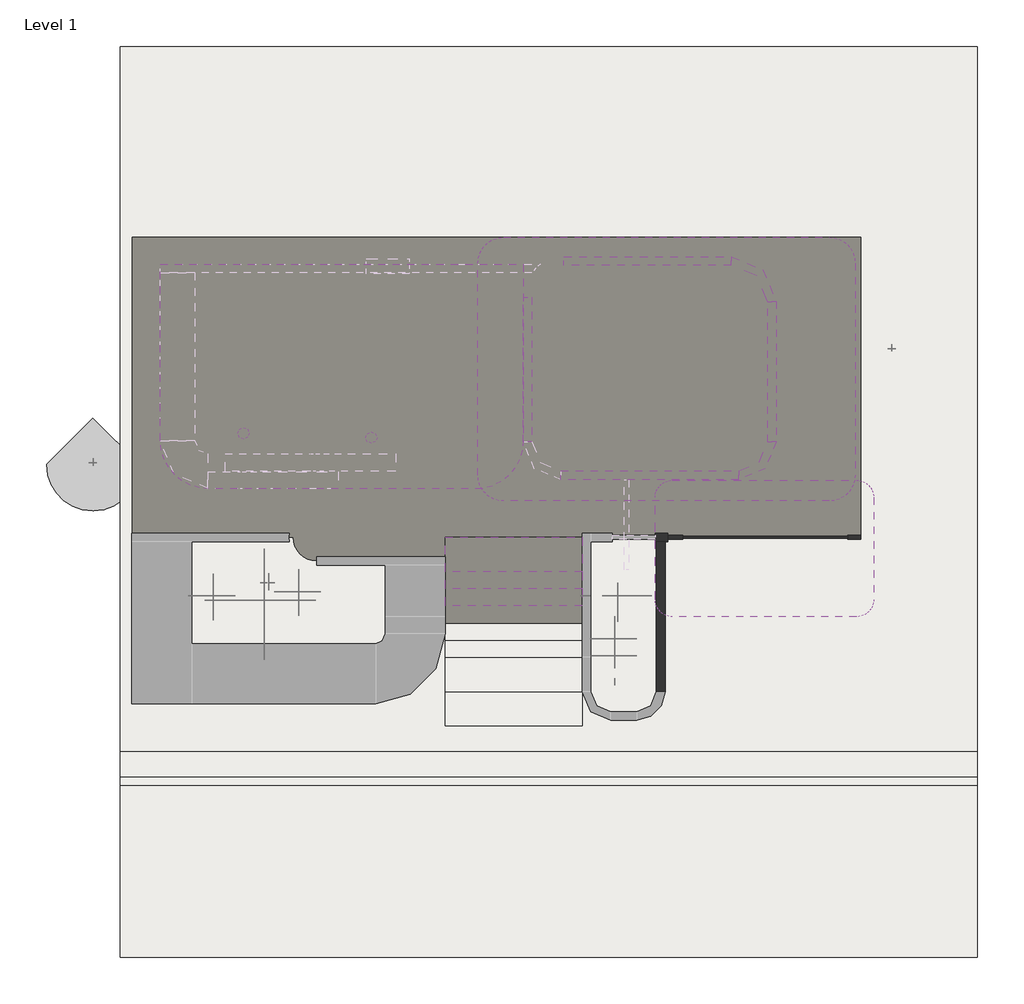
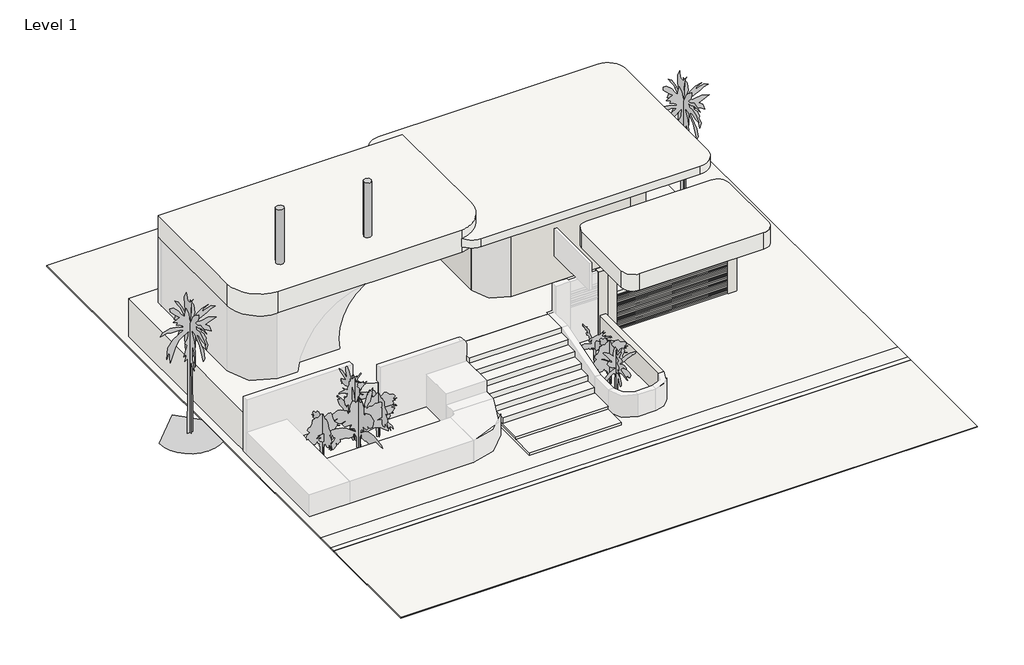
# One storey, part 2 of 2: 16 slabs, 12 walls, 9 geographic elements, 2 columns.
"""IFC4 building model written with IfcOpenShell, lengths in millimetres."""

from ifc_helpers import new_model, si_unit, point, frame, frame_2d, origin, origin_with_axes, place, context, project, spatial, polyline, circle_curve, trimmed, segment, composite_curve, outline, extrude, faceted_brep, transform, mapped, element, save
from components import column_386bdc77, rpc_tree_tropical_d7a905c7, rpc_tree_tropical_australian_tree_furn_6_77f1a640, rpc_tree_tropical_cuban_royal_palm_25_6f0ceb55, rpc_tree_tropical_golden_malay_palm_10_a310d7cf, rpc_tree_tropical_hurricane_palm_12_75f24be5, rpc_tree_tropical_japanese_fiber_banana_8_fc2fb2a9

model = new_model("IFC4")

# Units and contexts
model_context = context("Model", 3, world=origin())
ifc_project = project(units=[si_unit("LENGTHUNIT", "METRE", prefix="MILLI")], contexts=[model_context])

# Site, building, storey
site = spatial("IfcSite", under=ifc_project)
building = spatial("IfcBuilding", under=site)
storey = spatial("IfcBuildingStorey", under=building, Name="Level 1", Elevation=0.0)

# Columns
placement = place(None, origin())
column_shape = column_386bdc77(model_context)
element("IfcColumn", 1, ObjectType="Round Column.0001 : 06\" Diameter", at=placement, inside=storey, context=model_context, shape_type="MappedRepresentation", body=[
    mapped(column_shape, transform((-16218.3035766, 4084.0629979, 0.0), x_axis=(1.0, 0.0, 0.0), y_axis=(0.0, 1.0, 0.0), z_axis=(0.0, 0.0, 1.0))),
])
element("IfcColumn", 2, ObjectType="Round Column.0001 : 06\" Diameter", at=placement, inside=storey, context=model_context, shape_type="MappedRepresentation", body=[
    mapped(column_shape, transform((-11671.7035766, 3931.6629979, 0.0), x_axis=(1.0, 0.0, 0.0), y_axis=(0.0, 1.0, 0.0), z_axis=(0.0, 0.0, 1.0))),
])

# Geographic elements
rpc_tree_tropical_shape = rpc_tree_tropical_d7a905c7(model_context)
element("IfcGeographicElement", 3, ObjectType="RPC Tree - Tropical", at=placement, inside=storey, context=model_context, shape_type="MappedRepresentation", body=[
    mapped(rpc_tree_tropical_shape, transform((-15227.7035766, 3063.3953368, 0.0), x_axis=(1.0, 0.0, 0.0), y_axis=(0.0, 1.0, 0.0), z_axis=(0.0, 0.0, 1.0))),
])
element("IfcGeographicElement", 4, ObjectType="RPC Tree - Tropical", at=placement, inside=storey, context=model_context, shape_type="MappedRepresentation", body=[
    mapped(rpc_tree_tropical_shape, transform((-12179.7035766, 3215.7953368, 0.0), x_axis=(1.0, 0.0, 0.0), y_axis=(0.0, 1.0, 0.0), z_axis=(0.0, 0.0, 1.0))),
])
element("IfcGeographicElement", 5, ObjectType="RPC Tree - Tropical", at=placement, inside=storey, context=model_context, shape_type="MappedRepresentation", body=[
    mapped(rpc_tree_tropical_shape, transform((-936.864807, 1539.3953368, 0.0), x_axis=(1.0, 0.0, 0.0), y_axis=(0.0, 1.0, 0.0), z_axis=(0.0, 0.0, 1.0))),
])
rpc_tree_tropical_australian_tree_furn_6_shape = rpc_tree_tropical_australian_tree_furn_6_77f1a640(model_context)
element("IfcGeographicElement", 6, ObjectType="RPC Tree - Tropical : Australian Tree Furn - 6'", at=placement, inside=storey, context=model_context, shape_type="MappedRepresentation", body=[
    mapped(rpc_tree_tropical_australian_tree_furn_6_shape, transform((-828.8944013, 3063.3953368, 0.0), x_axis=(1.0, 0.0, 0.0), y_axis=(0.0, 1.0, 0.0), z_axis=(0.0, 0.0, 1.0))),
])
rpc_tree_tropical_cuban_royal_palm_25_shape = rpc_tree_tropical_cuban_royal_palm_25_6f0ceb55(model_context)
element("IfcGeographicElement", 7, ObjectType="RPC Tree - Tropical : Cuban Royal Palm - 25'", at=placement, inside=storey, context=model_context, shape_type="MappedRepresentation", body=[
    mapped(rpc_tree_tropical_cuban_royal_palm_25_shape, transform((-19494.9035766, 7787.7953368, 0.0), x_axis=(1.0, 0.0, 0.0), y_axis=(0.0, 1.0, 0.0), z_axis=(0.0, 0.0, 1.0))),
])
element("IfcGeographicElement", 8, ObjectType="RPC Tree - Tropical : Cuban Royal Palm - 25'", at=placement, inside=storey, context=model_context, shape_type="MappedRepresentation", body=[
    mapped(rpc_tree_tropical_cuban_royal_palm_25_shape, transform((8914.5561229, 11850.2999244, 0.0), x_axis=(1.0, 0.0, 0.0), y_axis=(0.0, 1.0, 0.0), z_axis=(0.0, 0.0, 1.0))),
])
rpc_tree_tropical_golden_malay_palm_10_shape = rpc_tree_tropical_golden_malay_palm_10_a310d7cf(model_context)
element("IfcGeographicElement", 9, ObjectType="RPC Tree - Tropical : Golden Malay Palm - 10'", at=placement, inside=storey, context=model_context, shape_type="MappedRepresentation", body=[
    mapped(rpc_tree_tropical_golden_malay_palm_10_shape, transform((-13398.9035766, 2910.9953368, 0.0), x_axis=(1.0, 0.0, 0.0), y_axis=(0.0, 1.0, 0.0), z_axis=(0.0, 0.0, 1.0))),
])
rpc_tree_tropical_hurricane_palm_12_shape = rpc_tree_tropical_hurricane_palm_12_75f24be5(model_context)
element("IfcGeographicElement", 10, ObjectType="RPC Tree - Tropical : Hurricane Palm - 12'", at=placement, inside=storey, context=model_context, shape_type="MappedRepresentation", body=[
    mapped(rpc_tree_tropical_hurricane_palm_12_shape, transform((-13246.5035766, 3520.5953368, 0.0), x_axis=(1.0, 0.0, 0.0), y_axis=(0.0, 1.0, 0.0), z_axis=(0.0, 0.0, 1.0))),
])
rpc_tree_tropical_japanese_fiber_banana_8_shape = rpc_tree_tropical_japanese_fiber_banana_8_fc2fb2a9(model_context)
element("IfcGeographicElement", 11, ObjectType="RPC Tree - Tropical : Japanese Fiber Banana - 8'", at=placement, inside=storey, context=model_context, shape_type="MappedRepresentation", body=[
    mapped(rpc_tree_tropical_japanese_fiber_banana_8_shape, transform((-936.864807, 929.7953368, 0.0), x_axis=(1.0, 0.0, 0.0), y_axis=(0.0, 1.0, 0.0), z_axis=(0.0, 0.0, 1.0))),
])

# Slabs
element("IfcSlab", 12, ObjectType="Generic - 1.5'", at=placement, inside=storey, context=model_context, shape_type="SweptSolid", body=[
    extrude(outline(composite_curve([segment(trimmed(circle_curve(frame_2d((6692.4964234, 14898.2999244)), 914.4), [point((6692.4964234, 15812.6999244))], [point((7606.8964234, 14898.2999244))], False, "CARTESIAN"), True, "CONTINUOUS"), segment(polyline([(7606.8964234, 14898.2999244), (7606.8964234, 7349.8857607)]), True, "CONTINUOUS"), segment(trimmed(circle_curve(frame_2d((6692.4964234, 7349.8857607)), 914.4), [point((7606.8964234, 7349.8857607))], [point((6692.4964234, 6435.4857607))], False, "CARTESIAN"), True, "CONTINUOUS"), segment(polyline([(6692.4964234, 6435.4857607), (-4890.8055301, 6435.4857607)]), True, "CONTINUOUS"), segment(trimmed(circle_curve(frame_2d((-4890.8055301, 7349.8857607)), 914.4), [point((-4890.8055301, 6435.4857607))], [point((-5805.2055301, 7349.8857607))], False, "CARTESIAN"), True, "CONTINUOUS"), segment(polyline([(-5805.2055301, 7349.8857607), (-5805.2055301, 14898.2999244)]), True, "CONTINUOUS"), segment(trimmed(circle_curve(frame_2d((-4890.8055301, 14898.2999244)), 914.4), [point((-5805.2055301, 14898.2999244))], [point((-4890.8055301, 15812.6999244))], False, "CARTESIAN"), True, "CONTINUOUS"), segment(polyline([(-4890.8055301, 15812.6999244), (6692.4964234, 15812.6999244)]), True, "CONTINUOUS")], self_intersect=False)), frame((0.0, 0.0, 6096.0), z_axis=(0.0, 0.0, 1.0), x_axis=(1.0, 0.0, 0.0)), (0.0, 0.0, 1.0), 457.2),
])
element("IfcSlab", 13, ObjectType="Generic - 12\"", at=placement, inside=storey, context=model_context, shape_type="SweptSolid", body=[
    extrude(outline(polyline([(-2097.7074836, 5144.6999244), (-2097.7074836, 877.4999244), (-6974.5074836, 877.4999244), (-6974.5074836, 5144.6999244), (-2097.7074836, 5144.6999244)])), frame((0.0, 0.0, 304.8), z_axis=(0.0, 0.0, 1.0), x_axis=(1.0, 0.0, 0.0)), (0.0, 0.0, 1.0), 304.8),
])
element("IfcSlab", 14, ObjectType="Generic - 12\"", at=placement, inside=storey, context=model_context, shape_type="SweptSolid", body=[
    extrude(outline(polyline([(-2097.7074836, 5144.6999244), (-2097.7074836, 1487.0999244), (-6974.5074836, 1487.0999244), (-6974.5074836, 5144.6999244), (-2097.7074836, 5144.6999244)])), frame((0.0, 0.0, 609.6), z_axis=(0.0, 0.0, 1.0), x_axis=(1.0, 0.0, 0.0)), (0.0, 0.0, 1.0), 304.8),
])
element("IfcSlab", 15, ObjectType="Generic - 12\"", at=placement, inside=storey, context=model_context, shape_type="SweptSolid", body=[
    extrude(outline(polyline([(-2097.7074836, 5144.6999244), (-2097.7074836, 2096.6999244), (-6974.5074836, 2096.6999244), (-6974.5074836, 5144.6999244), (-2097.7074836, 5144.6999244)])), frame((0.0, 0.0, 914.4), z_axis=(0.0, 0.0, 1.0), x_axis=(1.0, 0.0, 0.0)), (0.0, 0.0, 1.0), 304.8),
])
element("IfcSlab", 16, ObjectType="Generic - 12\"", at=placement, inside=storey, context=model_context, shape_type="SweptSolid", body=[
    extrude(outline(polyline([(-2097.7074836, 5144.6999244), (-2097.7074836, 2706.3092226), (-6974.5074836, 2706.3092226), (-6974.5074836, 5144.6999244), (-2097.7074836, 5144.6999244)])), frame((0.0, 0.0, 1219.2), z_axis=(0.0, 0.0, 1.0), x_axis=(1.0, 0.0, 0.0)), (0.0, 0.0, 1.0), 304.8),
])
element("IfcSlab", 17, ObjectType="Generic - 12\"", at=placement, inside=storey, context=model_context, shape_type="SweptSolid", body=[
    extrude(outline(polyline([(-2097.7074836, 5144.6999244), (-2097.7074836, 3315.8999244), (-6974.5074836, 3315.8999244), (-6974.5074836, 5144.6999244), (-2097.7074836, 5144.6999244)])), frame((0.0, 0.0, 1524.0), z_axis=(0.0, 0.0, 1.0), x_axis=(1.0, 0.0, 0.0)), (0.0, 0.0, 1.0), 304.8),
])
element("IfcSlab", 18, ObjectType="Generic - 12\"", at=placement, inside=storey, context=model_context, shape_type="SweptSolid", body=[
    extrude(outline(polyline([(-2097.7074836, 5144.6999244), (-2097.7074836, 3925.5045735), (-6974.5074836, 3925.5045735), (-6974.5074836, 5144.6999244), (-2097.7074836, 5144.6999244)])), frame((0.0, 0.0, 1828.8), z_axis=(0.0, 0.0, 1.0), x_axis=(1.0, 0.0, 0.0)), (0.0, 0.0, 1.0), 304.8),
])
element("IfcSlab", 19, ObjectType="Generic - 2\"", at=placement, inside=storey, context=model_context, shape_type="SweptSolid", body=[
    extrude(outline(polyline([(11957.1530585, 22597.74911), (11957.1530585, -2475.3000756), (-18522.8469415, -2475.3000756), (-18522.8469415, 22597.74911), (11957.1530585, 22597.74911)])), frame((0.0, 0.0, -50.8), z_axis=(0.0, 0.0, 1.0), x_axis=(1.0, 0.0, 0.0)), (0.0, 0.0, 1.0), 50.8),
])
element("IfcSlab", 20, ObjectType="Generic - 2\" gray", at=placement, inside=storey, context=model_context, shape_type="SweptSolid", body=[
    extrude(outline(polyline([(-18522.8469415, -2475.3000756), (11957.1530585, -2475.3000756), (11957.1530585, -3389.7000756), (-18522.8469415, -3389.7000756), (-18522.8469415, -2475.3000756)])), frame((0.0, 0.0, -50.8), z_axis=(0.0, 0.0, 1.0), x_axis=(1.0, 0.0, 0.0)), (0.0, 0.0, 1.0), 50.8),
])
element("IfcSlab", 21, ObjectType="Generic - 2\" gray", at=placement, inside=storey, context=model_context, shape_type="SweptSolid", body=[
    extrude(outline(polyline([(-18522.8469415, -3694.5000756), (11957.1530585, -3694.5000756), (11957.1530585, -9790.5000756), (-18522.8469415, -9790.5000756), (-18522.8469415, -3694.5000756)])), frame((0.0, 0.0, -50.8), z_axis=(0.0, 0.0, 1.0), x_axis=(1.0, 0.0, 0.0)), (0.0, 0.0, 1.0), 50.8),
])
element("IfcSlab", 22, ObjectType="Generic - 2\" white", at=placement, inside=storey, context=model_context, shape_type="SweptSolid", body=[
    extrude(outline(polyline([(-18522.8469415, -3389.7000756), (11957.1530585, -3389.7000756), (11957.1530585, -3694.5000756), (-18522.8469415, -3694.5000756), (-18522.8469415, -3389.7000756)])), frame((0.0, 0.0, -50.8), z_axis=(0.0, 0.0, 1.0), x_axis=(1.0, 0.0, 0.0)), (0.0, 0.0, 1.0), 50.8),
])
element("IfcSlab", 23, ObjectType="Generic - 3'", at=placement, inside=storey, context=model_context, shape_type="SweptSolid", body=[
    extrude(outline(composite_curve([segment(trimmed(circle_curve(frame_2d((7657.6964234, 6562.4857607)), 609.6), [point((7657.6964234, 7172.0857607))], [point((8267.2964234, 6562.4857607))], False, "CARTESIAN"), True, "CONTINUOUS"), segment(polyline([(8267.2964234, 6562.4857607), (8267.2964234, 2927.6793884)]), True, "CONTINUOUS"), segment(trimmed(circle_curve(frame_2d((7657.6964234, 2927.6793884)), 609.6), [point((8267.2964234, 2927.6793884))], [point((7657.6964234, 2318.0793884))], False, "CARTESIAN"), True, "CONTINUOUS"), segment(polyline([(7657.6964234, 2318.0793884), (1104.4964234, 2318.0793884)]), True, "CONTINUOUS"), segment(trimmed(circle_curve(frame_2d((1104.4964234, 2927.6793884)), 609.6), [point((1104.4964234, 2318.0793884))], [point((494.8964234, 2927.6793884))], False, "CARTESIAN"), True, "CONTINUOUS"), segment(polyline([(494.8964234, 2927.6793884), (494.8964234, 6562.4857607)]), True, "CONTINUOUS"), segment(trimmed(circle_curve(frame_2d((1104.4964234, 6562.4857607)), 609.6), [point((494.8964234, 6562.4857607))], [point((1104.4964234, 7172.0857607))], False, "CARTESIAN"), True, "CONTINUOUS"), segment(polyline([(1104.4964234, 7172.0857607), (7657.6964234, 7172.0857607)]), True, "CONTINUOUS")], self_intersect=False)), frame((0.0, 0.0, 4064.0), z_axis=(0.0, 0.0, 1.0), x_axis=(1.0, 0.0, 0.0)), (0.0, 0.0, 1.0), 914.4),
])
element("IfcSlab", 24, ObjectType="Generic - 3.5'", at=placement, inside=storey, context=model_context, shape_type="SweptSolid", body=[
    extrude(outline(composite_curve([segment(polyline([(-18097.9035766, 15812.6999244), (7808.2925164, 15812.6999244), (7808.2925164, 5144.6999244), (-6974.5074836, 5144.6999244), (-6974.5074836, 4309.74911), (-11546.5074836, 4309.74911)]), True, "CONTINUOUS"), segment(trimmed(circle_curve(frame_2d((-11546.5074836, 5144.6999244)), 834.9508144), [point((-11546.5074836, 4309.74911))], [point((-12381.458298, 5144.6999244))], False, "CARTESIAN"), True, "CONTINUOUS"), segment(polyline([(-12381.458298, 5144.6999244), (-18097.9035766, 5144.6999244), (-18097.9035766, 15812.6999244)]), True, "CONTINUOUS")], self_intersect=False)), origin_with_axes(), (0.0, 0.0, 1.0), 2133.6),
])
element("IfcSlab", 25, ObjectType="Generic - 5'", at=placement, inside=storey, context=model_context, shape_type="SweptSolid", body=[
    extrude(outline(composite_curve([segment(polyline([(-17097.1000691, 8579.8629979), (-17097.1000691, 14853.6629979), (-4191.8438771, 14853.6629979), (-4191.8438771, 8579.8629979)]), True, "CONTINUOUS"), segment(trimmed(circle_curve(frame_2d((-5921.3536308, 8579.8629979)), 1729.5097537), [point((-4191.8438771, 8579.8629979))], [point((-5637.4510356, 6873.8139644))], False, "CARTESIAN"), True, "CONTINUOUS"), segment(polyline([(-5637.4510356, 6873.8139644), (-15391.0510356, 6873.8139644)]), True, "CONTINUOUS"), segment(trimmed(circle_curve(frame_2d((-15391.0510356, 8579.8629979)), 1706.0490335), [point((-15391.0510356, 6873.8139644))], [point((-17097.1000691, 8579.8629979))], False, "CARTESIAN"), True, "CONTINUOUS")], self_intersect=False)), frame((0.0, 0.0, 5791.2), z_axis=(0.0, 0.0, 1.0), x_axis=(1.0, 0.0, 0.0)), (0.0, 0.0, 1.0), 1219.2),
])
element("IfcSlab", 26, ObjectType="Generic - 6\"", at=placement, inside=storey, context=model_context, shape_type="SweptSolid", body=[
    extrude(outline(polyline([(-2097.7074836, 5144.6999244), (-2097.7074836, -1560.9000756), (-6974.5074836, -1560.9000756), (-6974.5074836, 5144.6999244), (-2097.7074836, 5144.6999244)])), origin_with_axes(), (0.0, 0.0, 1.0), 152.4),
])
element("IfcSlab", 27, ObjectType="Generic - 6\"", at=placement, inside=storey, context=model_context, shape_type="SweptSolid", body=[
    extrude(outline(polyline([(-2097.7074836, 5144.6999244), (-2097.7074836, -341.7000756), (-6974.5074836, -341.7000756), (-6974.5074836, 5144.6999244), (-2097.7074836, 5144.6999244)])), frame((0.0, 0.0, 152.4), z_axis=(0.0, 0.0, 1.0), x_axis=(1.0, 0.0, 0.0)), (0.0, 0.0, 1.0), 152.4),
])

# Walls
element("IfcWall", 28, ObjectType="Generic - 12\" white", at=placement, inside=storey, context=model_context, shape_type="SweptSolid", body=[
    extrude(outline(polyline([(847.5055987, 4992.2999244), (847.5055987, -341.7000756), (542.7055987, -341.7000756), (542.7055987, 4992.2999244), (847.5055987, 4992.2999244)])), origin_with_axes(), (0.0, 0.0, 1.0), 1219.2),
])
element("IfcWall", 29, ObjectType="Generic - 12\" white", at=placement, inside=storey, context=model_context, shape_type="Brep", body=[
    faceted_brep([(494.8964234, 4992.2999244, 3657.6), (494.8964234, 4992.2999244, 0.0), (542.7055987, 4992.2999244, 0.0), (847.5055987, 4992.2999244, 0.0), (952.0964234, 4992.2999244, 0.0), (952.0964234, 4992.2999244, 3657.6), (494.8964234, 5297.0999244, 0.0), (494.8964234, 5297.0999244, 3657.6), (952.0964234, 5297.0999244, 3657.6), (952.0964234, 5297.0999244, 0.0), (494.8964234, 5068.4999244, 0.0), (494.8964234, 5220.8999244, 0.0), (952.0964234, 5220.8999244, 0.0), (952.0964234, 5068.4999244, 0.0)], [[[0, 1, 2, 3, 4, 5]], [[6, 7, 8, 9]], [[4, 3, 2, 1, 10, 11, 6, 9, 12, 13]], [[5, 4, 13, 12, 9, 8]], [[0, 5, 8, 7]], [[0, 7, 6, 11, 10, 1]]]),
])
element("IfcWall", 30, ObjectType="Generic - 12\" white", at=placement, inside=storey, context=model_context, shape_type="SweptSolid", body=[
    extrude(outline(polyline([(-3887.0438771, 13679.0999244), (-3887.0438771, 8537.6506138), (-4191.8438771, 8537.6506138), (-4191.8438771, 13679.0999244), (-3887.0438771, 13679.0999244)])), frame((0.0, 0.0, 2133.6), z_axis=(0.0, 0.0, 1.0), x_axis=(1.0, 0.0, 0.0)), (0.0, 0.0, 1.0), 3657.6),
])
element("IfcWall", 31, ObjectType="Generic - 12\" white", at=placement, inside=storey, context=model_context, shape_type="SweptSolid", body=[
    extrude(outline(polyline([(4494.9561229, 8537.6506138), (4494.9561229, 13522.2136873), (4799.7561229, 13522.2136873), (4799.7561229, 8537.6506138), (4494.9561229, 8537.6506138)])), frame((0.0, 0.0, 2133.6), z_axis=(0.0, 0.0, 1.0), x_axis=(1.0, 0.0, 0.0)), (0.0, 0.0, 1.0), 3962.4),
])
element("IfcWall", 32, ObjectType="Generic - 12\" white", at=placement, inside=storey, context=model_context, shape_type="SweptSolid", body=[
    extrude(outline(polyline([(-2746.2869957, 15124.6568058), (3197.3130043, 15124.6568058), (3197.3130043, 14819.8568058), (-2746.2869957, 14819.8568058), (-2746.2869957, 15124.6568058)])), frame((0.0, 0.0, 2133.6), z_axis=(0.0, 0.0, 1.0), x_axis=(1.0, 0.0, 0.0)), (0.0, 0.0, 1.0), 3962.4),
])
element("IfcWall", 33, ObjectType="Generic - 12\" white", at=placement, inside=storey, context=model_context, shape_type="SweptSolid", body=[
    extrude(outline(composite_curve([segment(polyline([(3461.9623149, 7199.8568058), (3461.9623149, 7504.6568058)]), True, "CONTINUOUS"), segment(trimmed(circle_curve(frame_2d((3461.9623149, 8537.6506138)), 1032.993808), [point((3461.9623149, 7504.6568058))], [point((4494.9561229, 8537.6506138))], True, "CARTESIAN"), True, "CONTINUOUS"), segment(polyline([(4494.9561229, 8537.6506138), (4799.7561229, 8537.6506138)]), True, "CONTINUOUS"), segment(trimmed(circle_curve(frame_2d((3461.9623149, 8537.6506138)), 1337.793808), [point((4799.7561229, 8537.6506138))], [point((3461.9623149, 7199.8568058))], False, "CARTESIAN"), True, "CONTINUOUS")], self_intersect=False)), frame((0.0, 0.0, 2133.6), z_axis=(0.0, 0.0, 1.0), x_axis=(1.0, 0.0, 0.0)), (0.0, 0.0, 1.0), 3962.4),
])
element("IfcWall", 34, ObjectType="Generic - 12\" white", at=placement, inside=storey, context=model_context, shape_type="SweptSolid", body=[
    extrude(outline(polyline([(-2854.0500691, 7504.6568058), (3461.9623149, 7504.6568058), (3461.9623149, 7199.8568058), (-2854.0500691, 7199.8568058), (-2854.0500691, 7504.6568058)])), frame((0.0, 0.0, 2133.6), z_axis=(0.0, 0.0, 1.0), x_axis=(1.0, 0.0, 0.0)), (0.0, 0.0, 1.0), 3962.4),
])
element("IfcWall", 35, ObjectType="Generic - 12\" white", at=placement, inside=storey, context=model_context, shape_type="SweptSolid", body=[
    extrude(outline(composite_curve([segment(polyline([(4799.7561229, 13522.2136873), (4494.9561229, 13522.2136873)]), True, "CONTINUOUS"), segment(trimmed(circle_curve(frame_2d((3197.3130043, 13522.2136873)), 1297.6431186), [point((4494.9561229, 13522.2136873))], [point((3197.3130043, 14819.8568058))], True, "CARTESIAN"), True, "CONTINUOUS"), segment(polyline([(3197.3130043, 14819.8568058), (3197.3130043, 15124.6568058)]), True, "CONTINUOUS"), segment(trimmed(circle_curve(frame_2d((3197.3130043, 13522.2136873)), 1602.4431186), [point((3197.3130043, 15124.6568058))], [point((4799.7561229, 13522.2136873))], False, "CARTESIAN"), True, "CONTINUOUS")], self_intersect=False)), frame((0.0, 0.0, 2133.6), z_axis=(0.0, 0.0, 1.0), x_axis=(1.0, 0.0, 0.0)), (0.0, 0.0, 1.0), 3962.4),
])
element("IfcWall", 36, ObjectType="Generic - 3\" white 2", at=placement, inside=storey, context=model_context, shape_type="SweptSolid", body=[
    extrude(outline(polyline([(7352.8964234, 5106.5999244), (1468.8829427, 5106.5999244), (1468.8829427, 5182.7999244), (7352.8964234, 5182.7999244), (7352.8964234, 5106.5999244)])), origin_with_axes(), (0.0, 0.0, 1.0), 76.2),
    extrude(outline(polyline([(7352.8964234, 5106.5999244), (1468.8829427, 5106.5999244), (1468.8829427, 5182.7999244), (7352.8964234, 5182.7999244), (7352.8964234, 5106.5999244)])), frame((0.0, 0.0, 88.9), z_axis=(0.0, 0.0, 1.0), x_axis=(1.0, 0.0, 0.0)), (0.0, 0.0, 1.0), 76.2),
    extrude(outline(polyline([(7352.8964234, 5106.5999244), (1468.8829427, 5106.5999244), (1468.8829427, 5182.7999244), (7352.8964234, 5182.7999244), (7352.8964234, 5106.5999244)])), frame((0.0, 0.0, 177.8), z_axis=(0.0, 0.0, 1.0), x_axis=(1.0, 0.0, 0.0)), (0.0, 0.0, 1.0), 76.2),
    extrude(outline(polyline([(7352.8964234, 5106.5999244), (1468.8829427, 5106.5999244), (1468.8829427, 5182.7999244), (7352.8964234, 5182.7999244), (7352.8964234, 5106.5999244)])), frame((0.0, 0.0, 266.7), z_axis=(0.0, 0.0, 1.0), x_axis=(1.0, 0.0, 0.0)), (0.0, 0.0, 1.0), 76.2),
    extrude(outline(polyline([(7352.8964234, 5106.5999244), (1468.8829427, 5106.5999244), (1468.8829427, 5182.7999244), (7352.8964234, 5182.7999244), (7352.8964234, 5106.5999244)])), frame((0.0, 0.0, 355.6), z_axis=(0.0, 0.0, 1.0), x_axis=(1.0, 0.0, 0.0)), (0.0, 0.0, 1.0), 76.2),
    extrude(outline(polyline([(7352.8964234, 5106.5999244), (1468.8829427, 5106.5999244), (1468.8829427, 5182.7999244), (7352.8964234, 5182.7999244), (7352.8964234, 5106.5999244)])), frame((0.0, 0.0, 444.5), z_axis=(0.0, 0.0, 1.0), x_axis=(1.0, 0.0, 0.0)), (0.0, 0.0, 1.0), 76.2),
    extrude(outline(polyline([(7352.8964234, 5106.5999244), (1468.8829427, 5106.5999244), (1468.8829427, 5182.7999244), (7352.8964234, 5182.7999244), (7352.8964234, 5106.5999244)])), frame((0.0, 0.0, 533.4), z_axis=(0.0, 0.0, 1.0), x_axis=(1.0, 0.0, 0.0)), (0.0, 0.0, 1.0), 76.2),
    extrude(outline(polyline([(7352.8964234, 5106.5999244), (1468.8829427, 5106.5999244), (1468.8829427, 5182.7999244), (7352.8964234, 5182.7999244), (7352.8964234, 5106.5999244)])), frame((0.0, 0.0, 622.3), z_axis=(0.0, 0.0, 1.0), x_axis=(1.0, 0.0, 0.0)), (0.0, 0.0, 1.0), 76.2),
    extrude(outline(polyline([(7352.8964234, 5106.5999244), (1468.8829427, 5106.5999244), (1468.8829427, 5182.7999244), (7352.8964234, 5182.7999244), (7352.8964234, 5106.5999244)])), frame((0.0, 0.0, 711.2), z_axis=(0.0, 0.0, 1.0), x_axis=(1.0, 0.0, 0.0)), (0.0, 0.0, 1.0), 76.2),
    extrude(outline(polyline([(7352.8964234, 5106.5999244), (1468.8829427, 5106.5999244), (1468.8829427, 5182.7999244), (7352.8964234, 5182.7999244), (7352.8964234, 5106.5999244)])), frame((0.0, 0.0, 800.1), z_axis=(0.0, 0.0, 1.0), x_axis=(1.0, 0.0, 0.0)), (0.0, 0.0, 1.0), 76.2),
    extrude(outline(polyline([(7352.8964234, 5106.5999244), (1468.8829427, 5106.5999244), (1468.8829427, 5182.7999244), (7352.8964234, 5182.7999244), (7352.8964234, 5106.5999244)])), frame((0.0, 0.0, 889.0), z_axis=(0.0, 0.0, 1.0), x_axis=(1.0, 0.0, 0.0)), (0.0, 0.0, 1.0), 76.2),
])
element("IfcWall", 37, ObjectType="Generic - 3\" white 2", at=placement, inside=storey, context=model_context, shape_type="SweptSolid", body=[
    extrude(outline(polyline([(7352.8964234, 5106.5999244), (1468.8829427, 5106.5999244), (1468.8829427, 5182.7999244), (7352.8964234, 5182.7999244), (7352.8964234, 5106.5999244)])), frame((0.0, 0.0, 987.425), z_axis=(0.0, 0.0, 1.0), x_axis=(1.0, 0.0, 0.0)), (0.0, 0.0, 1.0), 76.2),
    extrude(outline(polyline([(7352.8964234, 5106.5999244), (1468.8829427, 5106.5999244), (1468.8829427, 5182.7999244), (7352.8964234, 5182.7999244), (7352.8964234, 5106.5999244)])), frame((0.0, 0.0, 1076.325), z_axis=(0.0, 0.0, 1.0), x_axis=(1.0, 0.0, 0.0)), (0.0, 0.0, 1.0), 76.2),
    extrude(outline(polyline([(7352.8964234, 5106.5999244), (1468.8829427, 5106.5999244), (1468.8829427, 5182.7999244), (7352.8964234, 5182.7999244), (7352.8964234, 5106.5999244)])), frame((0.0, 0.0, 1165.225), z_axis=(0.0, 0.0, 1.0), x_axis=(1.0, 0.0, 0.0)), (0.0, 0.0, 1.0), 76.2),
    extrude(outline(polyline([(7352.8964234, 5106.5999244), (1468.8829427, 5106.5999244), (1468.8829427, 5182.7999244), (7352.8964234, 5182.7999244), (7352.8964234, 5106.5999244)])), frame((0.0, 0.0, 1254.125), z_axis=(0.0, 0.0, 1.0), x_axis=(1.0, 0.0, 0.0)), (0.0, 0.0, 1.0), 76.2),
    extrude(outline(polyline([(7352.8964234, 5106.5999244), (1468.8829427, 5106.5999244), (1468.8829427, 5182.7999244), (7352.8964234, 5182.7999244), (7352.8964234, 5106.5999244)])), frame((0.0, 0.0, 1343.025), z_axis=(0.0, 0.0, 1.0), x_axis=(1.0, 0.0, 0.0)), (0.0, 0.0, 1.0), 76.2),
    extrude(outline(polyline([(7352.8964234, 5106.5999244), (1468.8829427, 5106.5999244), (1468.8829427, 5182.7999244), (7352.8964234, 5182.7999244), (7352.8964234, 5106.5999244)])), frame((0.0, 0.0, 1431.925), z_axis=(0.0, 0.0, 1.0), x_axis=(1.0, 0.0, 0.0)), (0.0, 0.0, 1.0), 76.2),
    extrude(outline(polyline([(7352.8964234, 5106.5999244), (1468.8829427, 5106.5999244), (1468.8829427, 5182.7999244), (7352.8964234, 5182.7999244), (7352.8964234, 5106.5999244)])), frame((0.0, 0.0, 1520.825), z_axis=(0.0, 0.0, 1.0), x_axis=(1.0, 0.0, 0.0)), (0.0, 0.0, 1.0), 76.2),
    extrude(outline(polyline([(7352.8964234, 5106.5999244), (1468.8829427, 5106.5999244), (1468.8829427, 5182.7999244), (7352.8964234, 5182.7999244), (7352.8964234, 5106.5999244)])), frame((0.0, 0.0, 1609.725), z_axis=(0.0, 0.0, 1.0), x_axis=(1.0, 0.0, 0.0)), (0.0, 0.0, 1.0), 76.2),
    extrude(outline(polyline([(7352.8964234, 5106.5999244), (1468.8829427, 5106.5999244), (1468.8829427, 5182.7999244), (7352.8964234, 5182.7999244), (7352.8964234, 5106.5999244)])), frame((0.0, 0.0, 1698.625), z_axis=(0.0, 0.0, 1.0), x_axis=(1.0, 0.0, 0.0)), (0.0, 0.0, 1.0), 76.2),
    extrude(outline(polyline([(7352.8964234, 5106.5999244), (1468.8829427, 5106.5999244), (1468.8829427, 5182.7999244), (7352.8964234, 5182.7999244), (7352.8964234, 5106.5999244)])), frame((0.0, 0.0, 1787.525), z_axis=(0.0, 0.0, 1.0), x_axis=(1.0, 0.0, 0.0)), (0.0, 0.0, 1.0), 76.2),
    extrude(outline(polyline([(7352.8964234, 5106.5999244), (1468.8829427, 5106.5999244), (1468.8829427, 5182.7999244), (7352.8964234, 5182.7999244), (7352.8964234, 5106.5999244)])), frame((0.0, 0.0, 1876.425), z_axis=(0.0, 0.0, 1.0), x_axis=(1.0, 0.0, 0.0)), (0.0, 0.0, 1.0), 76.2),
])
element("IfcWall", 38, ObjectType="Generic - 6\" white", at=placement, inside=storey, context=model_context, shape_type="Brep", body=[
    faceted_brep([(952.0964234, 5068.4999244, 0.0), (1468.8829427, 5068.4999244, 0.0), (1468.8829427, 5068.4999244, 4876.8), (952.0964234, 5068.4999244, 4876.8), (952.0964234, 5220.8999244, 0.0), (952.0964234, 5220.8999244, 4876.8), (1468.8829427, 5220.8999244, 4876.8), (1468.8829427, 5220.8999244, 0.0), (1468.8829427, 5182.7999244, 0.0), (1468.8829427, 5106.5999244, 0.0)], [[[0, 1, 2, 3]], [[4, 5, 6, 7]], [[1, 0, 4, 7, 8, 9]], [[3, 2, 6, 5]], [[0, 3, 5, 4]], [[1, 9, 8, 7, 6, 2]]]),
])
element("IfcWall", 39, ObjectType="Generic - 6\" white", at=placement, inside=storey, context=model_context, shape_type="Brep", body=[
    faceted_brep([(7352.8964234, 5068.4999244, 4876.8), (7352.8964234, 5068.4999244, 0.0), (7810.0964234, 5068.4999244, 0.0), (7810.0964234, 5068.4999244, 4876.8), (7352.8964234, 5220.8999244, 0.0), (7352.8964234, 5220.8999244, 4876.8), (7810.0964234, 5220.8999244, 4876.8), (7810.0964234, 5220.8999244, 0.0), (7352.8964234, 5106.5999244, 0.0), (7352.8964234, 5182.7999244, 0.0)], [[[0, 1, 2, 3]], [[4, 5, 6, 7]], [[2, 1, 8, 9, 4, 7]], [[3, 2, 7, 6]], [[0, 3, 6, 5]], [[0, 5, 4, 9, 8, 1]]]),
])

save(model, "model.ifc")

# Revit data of these elements
# Type "Round Column.0001 : 06\" Diameter"
#   Assembly Code = "B1010200"
#   Diameter = 1' - 0"
#   Offset Base = 0' - 0"
#   Offset Top = 0' - 0"
#   Material = EIFS, Exterior Insulation
# Type "RPC Tree - Tropical"
#   built-in parameter 1005198 = "{2, 15},{39, RPC-16-G2MF-J1Q0-CAN1-N000-ST1L-LVER-AU},{1, 0},{1, 0},{2, 13},{1, 8},{5, Color},{1, 0},{1, 0},{3, 0.8},{3, 0.8},{3, 0.8},{1, 8},{7, BBoxMin},{1, 0},{1, 0},{1, 0},{1, 0},{1, 0},{1, 8},{7, BBoxMax},{1, 0},{1, 0},{1, 0},{1, 0},{1, 0},{2, 11},{9, RPCTypeId},{1, 0},{1, 0},{39, RPC-16-G2MF-J1Q0-CAN1-N000-ST1L-LVER-AU},{1, 6},{14, RPCPlantHeight},{1, 0},{1, 0},{1, 8},{2, 11},{7, keyword},{1, 0},{1, 0},{35, :RPCs:Trees [Tropical]:Geometry:RPC},{2, 11},{8, category},{1, 0},{1, 0},{16, Trees [Tropical]},{2, 11},{12, LocalizedUID},{1, 0},{1, 0},{13, Windmill Palm},{2, 14},{6, Height},{1, 0},{1, 0},{1, 8},{1, 2},{16, Cast Reflections},{1, 0},{1, 0},{1, 0},{1, 2},{12, Cast Shadows},{1, 0},{1, 0},{1, 1},{1, 2},{9, Lock View},{1, 0},{1, 0},{1, 0},{1, 4},{5, ViewC},{1, 0},{1, 0},{1, 0},{21, assetlibrary_base.fbx},{1, 5},"
#   built-in parameter 1005195 = "RPC-16-G2MF-J1Q0-CAN1-N000-ST1L-LVER-AU"
#   Assembly Code = "G2050500"
#   Height = 8' - 0"
#   Plan Symbol = element 387627
#   Default Elevation = 0
# Type "RPC Tree - Tropical : Australian Tree Furn - 6'"
#   built-in parameter 1005198 = "{2, 15},{39, RPC-16-FVCN-UWG0-AP53-A000-ST1L-LVER-AU},{1, 0},{1, 0},{2, 13},{1, 8},{5, Color},{1, 0},{1, 0},{3, 0.8},{3, 0.8},{3, 0.8},{1, 8},{7, BBoxMin},{1, 0},{1, 0},{1, 0},{1, 0},{1, 0},{1, 8},{7, BBoxMax},{1, 0},{1, 0},{1, 0},{1, 0},{1, 0},{2, 11},{9, RPCTypeId},{1, 0},{1, 0},{39, RPC-16-FVCN-UWG0-AP53-A000-ST1L-LVER-AU},{1, 6},{14, RPCPlantHeight},{1, 0},{1, 0},{1, 6},{2, 11},{7, keyword},{1, 0},{1, 0},{35, :RPCs:Trees [Tropical]:Geometry:RPC},{2, 11},{8, category},{1, 0},{1, 0},{16, Trees [Tropical]},{2, 11},{12, LocalizedUID},{1, 0},{1, 0},{20, Australian Tree Fern},{2, 14},{6, Height},{1, 0},{1, 0},{1, 6},{1, 2},{16, Cast Reflections},{1, 0},{1, 0},{1, 0},{1, 2},{12, Cast Shadows},{1, 0},{1, 0},{1, 1},{1, 2},{9, Lock View},{1, 0},{1, 0},{1, 0},{1, 4},{5, ViewC},{1, 0},{1, 0},{1, 0},{21, assetlibrary_base.fbx},{1, 5},"
#   built-in parameter 1005195 = "RPC-16-FVCN-UWG0-AP53-A000-ST1L-LVER-AU"
#   Type Comments = "Australian Tree Furn"
#   Assembly Code = "G2050500"
#   Height = 6' - 0"
#   Plan Symbol = element 387627
#   Default Elevation = 0
# Type "RPC Tree - Tropical : Cuban Royal Palm - 25'"
#   built-in parameter 1005198 = "{2, 15},{39, RPC-16-FVGV-NKG0-7NHH-C000-ST1L-LVER-AU},{1, 0},{1, 0},{2, 13},{1, 8},{5, Color},{1, 0},{1, 0},{3, 0.8},{3, 0.8},{3, 0.8},{1, 8},{7, BBoxMin},{1, 0},{1, 0},{1, 0},{1, 0},{1, 0},{1, 8},{7, BBoxMax},{1, 0},{1, 0},{1, 0},{1, 0},{1, 0},{2, 11},{9, RPCTypeId},{1, 0},{1, 0},{39, RPC-16-FVGV-NKG0-7NHH-C000-ST1L-LVER-AU},{1, 6},{14, RPCPlantHeight},{1, 0},{1, 0},{2, 25},{2, 11},{7, keyword},{1, 0},{1, 0},{35, :RPCs:Trees [Tropical]:Geometry:RPC},{2, 11},{8, category},{1, 0},{1, 0},{16, Trees [Tropical]},{2, 11},{12, LocalizedUID},{1, 0},{1, 0},{16, Cuban Royal Palm},{2, 14},{6, Height},{1, 0},{1, 0},{2, 25},{1, 2},{16, Cast Reflections},{1, 0},{1, 0},{1, 0},{1, 2},{12, Cast Shadows},{1, 0},{1, 0},{1, 1},{1, 2},{9, Lock View},{1, 0},{1, 0},{1, 0},{1, 4},{5, ViewC},{1, 0},{1, 0},{1, 0},{21, assetlibrary_base.fbx},{1, 5},"
#   built-in parameter 1005195 = "RPC-16-FVGV-NKG0-7NHH-C000-ST1L-LVER-AU"
#   Type Comments = "Cuban Royal Palm"
#   Assembly Code = "G2050500"
#   Height = 25' - 0"
#   Plan Symbol = element 387627
#   Default Elevation = 0
# Type "RPC Tree - Tropical : Golden Malay Palm - 10'"
#   built-in parameter 1005198 = "{2, 15},{39, RPC-16-FXGM-2RXX-PGXL-E000-ST1L-LVER-AU},{1, 0},{1, 0},{2, 13},{1, 8},{5, Color},{1, 0},{1, 0},{3, 0.8},{3, 0.8},{3, 0.8},{1, 8},{7, BBoxMin},{1, 0},{1, 0},{1, 0},{1, 0},{1, 0},{1, 8},{7, BBoxMax},{1, 0},{1, 0},{1, 0},{1, 0},{1, 0},{2, 11},{9, RPCTypeId},{1, 0},{1, 0},{39, RPC-16-FXGM-2RXX-PGXL-E000-ST1L-LVER-AU},{1, 6},{14, RPCPlantHeight},{1, 0},{1, 0},{2, 10},{2, 11},{7, keyword},{1, 0},{1, 0},{35, :RPCs:Trees [Tropical]:Geometry:RPC},{2, 11},{8, category},{1, 0},{1, 0},{16, Trees [Tropical]},{2, 11},{12, LocalizedUID},{1, 0},{1, 0},{17, Golden Malay Palm},{2, 14},{6, Height},{1, 0},{1, 0},{2, 10},{1, 2},{16, Cast Reflections},{1, 0},{1, 0},{1, 0},{1, 2},{12, Cast Shadows},{1, 0},{1, 0},{1, 1},{1, 2},{9, Lock View},{1, 0},{1, 0},{1, 0},{1, 4},{5, ViewC},{1, 0},{1, 0},{1, 0},{21, assetlibrary_base.fbx},{1, 5},"
#   built-in parameter 1005195 = "RPC-16-FXGM-2RXX-PGXL-E000-ST1L-LVER-AU"
#   Type Comments = "Golden Malay Palm"
#   Assembly Code = "G2050500"
#   Height = 10' - 0"
#   Plan Symbol = element 387627
#   Default Elevation = 0
# Type "RPC Tree - Tropical : Hurricane Palm - 12'"
#   built-in parameter 1005198 = "{2, 15},{39, RPC-16-FXGL-UL7X-PH44-0000-ST1L-LVER-AU},{1, 0},{1, 0},{2, 13},{1, 8},{5, Color},{1, 0},{1, 0},{3, 0.8},{3, 0.8},{3, 0.8},{1, 8},{7, BBoxMin},{1, 0},{1, 0},{1, 0},{1, 0},{1, 0},{1, 8},{7, BBoxMax},{1, 0},{1, 0},{1, 0},{1, 0},{1, 0},{2, 11},{9, RPCTypeId},{1, 0},{1, 0},{39, RPC-16-FXGL-UL7X-PH44-0000-ST1L-LVER-AU},{1, 6},{14, RPCPlantHeight},{1, 0},{1, 0},{2, 12},{2, 11},{7, keyword},{1, 0},{1, 0},{35, :RPCs:Trees [Tropical]:Geometry:RPC},{2, 11},{8, category},{1, 0},{1, 0},{16, Trees [Tropical]},{2, 11},{12, LocalizedUID},{1, 0},{1, 0},{14, Hurricane Palm},{2, 14},{6, Height},{1, 0},{1, 0},{2, 12},{1, 2},{16, Cast Reflections},{1, 0},{1, 0},{1, 0},{1, 2},{12, Cast Shadows},{1, 0},{1, 0},{1, 1},{1, 2},{9, Lock View},{1, 0},{1, 0},{1, 0},{1, 4},{5, ViewC},{1, 0},{1, 0},{1, 0},{21, assetlibrary_base.fbx},{1, 5},"
#   built-in parameter 1005195 = "RPC-16-FXGL-UL7X-PH44-0000-ST1L-LVER-AU"
#   Type Comments = "Hurricane Palm"
#   Assembly Code = "G2050500"
#   Height = 12' - 0"
#   Plan Symbol = element 387627
#   Default Elevation = 0
# Type "RPC Tree - Tropical : Japanese Fiber Banana - 8'"
#   built-in parameter 1005198 = "{2, 15},{39, RPC-16-FVGT-NR7X-7G1M-A000-ST1L-LVER-AU},{1, 0},{1, 0},{2, 13},{1, 8},{5, Color},{1, 0},{1, 0},{3, 0.8},{3, 0.8},{3, 0.8},{1, 8},{7, BBoxMin},{1, 0},{1, 0},{1, 0},{1, 0},{1, 0},{1, 8},{7, BBoxMax},{1, 0},{1, 0},{1, 0},{1, 0},{1, 0},{2, 11},{9, RPCTypeId},{1, 0},{1, 0},{39, RPC-16-FVGT-NR7X-7G1M-A000-ST1L-LVER-AU},{1, 6},{14, RPCPlantHeight},{1, 0},{1, 0},{1, 8},{2, 11},{7, keyword},{1, 0},{1, 0},{35, :RPCs:Trees [Tropical]:Geometry:RPC},{2, 11},{8, category},{1, 0},{1, 0},{16, Trees [Tropical]},{2, 11},{12, LocalizedUID},{1, 0},{1, 0},{21, Japanese Fiber Banana},{2, 14},{6, Height},{1, 0},{1, 0},{1, 8},{1, 2},{16, Cast Reflections},{1, 0},{1, 0},{1, 0},{1, 2},{12, Cast Shadows},{1, 0},{1, 0},{1, 1},{1, 2},{9, Lock View},{1, 0},{1, 0},{1, 0},{1, 4},{5, ViewC},{1, 0},{1, 0},{1, 0},{21, assetlibrary_base.fbx},{1, 5},"
#   built-in parameter 1005195 = "RPC-16-FVGT-NR7X-7G1M-A000-ST1L-LVER-AU"
#   Type Comments = "Japanese Fiber Banana"
#   Assembly Code = "G2050500"
#   Height = 8' - 0"
#   Plan Symbol = element 387627
#   Default Elevation = 0
# Type "Generic - 1.5'"
#   Assembly Code = "B1010"
#   Function = 0
#   Layers, outside or top first: 1' - 6" "Door - Frame" (function 1)
# Type "Generic - 12\""
#   Assembly Code = "B1010"
#   Function = 0
#   Layers, outside or top first: 1' - 0" "Door - Frame" (function 1)
# Type "Generic - 2\""
#   Assembly Code = "B1010"
#   Function = 0
#   Layers, outside or top first: 0' - 2" "Damp-proofing" (function 1)
# Type "Generic - 2\" gray"
#   Assembly Code = "B1010"
#   Function = 0
#   Layers, outside or top first: 0' - 2" "Concrete, Cast-in-Place gray" (function 1)
# Type "Generic - 2\" white"
#   Assembly Code = "B1010"
#   Function = 0
#   Layers, outside or top first: 0' - 2" "Door - Frame" (function 1)
# Type "Generic - 3'"
#   Assembly Code = "B1010"
#   Function = 0
#   Layers, outside or top first: 3' - 0" "Door - Frame" (function 1)
# Type "Generic - 3.5'"
#   Assembly Code = "B1010"
#   Function = 0
#   Layers, outside or top first: 7' - 0" "Door - Frame" (function 1)
# Type "Generic - 5'"
#   Assembly Code = "B1010"
#   Function = 0
#   Layers, outside or top first: 4' - 0" "Door - Frame" (function 1)
# Type "Generic - 6\""
#   Assembly Code = "B1010"
#   Function = 0
#   Layers, outside or top first: 0' - 6" "Door - Frame" (function 1)
# Type "Generic - 12\" white"
#   Assembly Code = "B2010"
#   Layers, outside or top first: 1' - 0" "Door - Frame" (function 1)
# Type "Generic - 3\" white 2"
#   Assembly Code = "B2010"
#   Layers, outside or top first: 0' - 3" "Door - Frame" (function 1)
# Type "Generic - 6\" white"
#   Assembly Code = "B2010"
#   Layers, outside or top first: 0' - 6" "Door - Frame" (function 1)
# Elements 1, 2 (IfcColumn, "Round Column.0001 : 06\" Diameter")
#   Phase Created = New Construction
# Elements 3, 4, 5 (IfcGeographicElement, "RPC Tree - Tropical")
#   Phase Created = New Construction
# Element 6 (IfcGeographicElement, "RPC Tree - Tropical : Australian Tree Furn - 6'")
#   Phase Created = New Construction
# Elements 7, 8 (IfcGeographicElement, "RPC Tree - Tropical : Cuban Royal Palm - 25'")
#   Phase Created = New Construction
# Element 9 (IfcGeographicElement, "RPC Tree - Tropical : Golden Malay Palm - 10'")
#   Phase Created = New Construction
# Element 10 (IfcGeographicElement, "RPC Tree - Tropical : Hurricane Palm - 12'")
#   Phase Created = New Construction
# Element 11 (IfcGeographicElement, "RPC Tree - Tropical : Japanese Fiber Banana - 8'")
#   Phase Created = New Construction
# Element 12 (IfcSlab, "Generic - 1.5'")
#   Height Offset From Level = 21' - 6"
#   Phase Created = New Construction
#   Materials on its faces: "Door - Frame"
# Element 13 (IfcSlab, "Generic - 12\"")
#   Height Offset From Level = 2' - 0"
#   Phase Created = New Construction
#   Materials on its faces: "Door - Frame"
# Element 14 (IfcSlab, "Generic - 12\"")
#   Height Offset From Level = 3' - 0"
#   Phase Created = New Construction
#   Materials on its faces: "Door - Frame"
# Element 15 (IfcSlab, "Generic - 12\"")
#   Height Offset From Level = 4' - 0"
#   Phase Created = New Construction
#   Materials on its faces: "Door - Frame"
# Element 16 (IfcSlab, "Generic - 12\"")
#   Height Offset From Level = 5' - 0"
#   Phase Created = New Construction
#   Materials on its faces: "Door - Frame"
# Element 17 (IfcSlab, "Generic - 12\"")
#   Height Offset From Level = 6' - 0"
#   Phase Created = New Construction
#   Materials on its faces: "Door - Frame"
# Element 18 (IfcSlab, "Generic - 12\"")
#   Height Offset From Level = 7' - 0"
#   Phase Created = New Construction
#   Materials on its faces: "Door - Frame"
# Element 19 (IfcSlab, "Generic - 2\"")
#   Height Offset From Level = 0' - 0"
#   Phase Created = New Construction
#   Materials on its faces: "Damp-proofing"
# Elements 20, 21 (IfcSlab, "Generic - 2\" gray")
#   built-in parameter 1001955 = 3.14159 (stored number, unit not read)
#   Height Offset From Level = 0' - 0"
#   Phase Created = New Construction
#   Materials on its faces: "Concrete, Cast-in-Place gray"
# Element 22 (IfcSlab, "Generic - 2\" white")
#   built-in parameter 1001955 = 3.14159 (stored number, unit not read)
#   Height Offset From Level = 0' - 0"
#   Phase Created = New Construction
#   Materials on its faces: "Door - Frame"
# Element 23 (IfcSlab, "Generic - 3'")
#   Height Offset From Level = 16' - 4"
#   Phase Created = New Construction
#   Materials on its faces: "Door - Frame"
# Element 24 (IfcSlab, "Generic - 3.5'")
#   built-in parameter 1001955 = 3.14159 (stored number, unit not read)
#   Height Offset From Level = 7' - 0"
#   Phase Created = New Construction
#   Materials on its faces: "Door - Frame"
# Element 25 (IfcSlab, "Generic - 5'")
#   Height Offset From Level = 23' - 0"
#   Phase Created = New Construction
#   Materials on its faces: "Door - Frame"
# Element 26 (IfcSlab, "Generic - 6\"")
#   Height Offset From Level = 0' - 6"
#   Phase Created = New Construction
#   Materials on its faces: "Door - Frame"
# Element 27 (IfcSlab, "Generic - 6\"")
#   Height Offset From Level = 1' - 0"
#   Phase Created = New Construction
#   Materials on its faces: "Door - Frame"
# Element 28 (IfcWall, "Generic - 12\" white")
#   Top Offset = 0' - 0"
#   Base Offset = 0' - 0"
#   Unconnected Height = 4' - 0"
#   wall height = 4' - 0"
#   Phase Created = New Construction
#   Base Constraint = Level 1
#   Materials on its faces: "Door - Frame"
# Element 29 (IfcWall, "Generic - 12\" white")
#   Top Offset = 0' - 0"
#   Base Offset = 0' - 0"
#   Unconnected Height = 12' - 0"
#   wall height = 12' - 0"
#   Phase Created = New Construction
#   Base Constraint = Level 1
#   Materials on its faces: "Door - Frame"
# Element 30 (IfcWall, "Generic - 12\" white")
#   built-in parameter 1001111 = 7' - 0"
#   Top Offset = 0' - 0"
#   Base Offset = 7' - 0"
#   Unconnected Height = 12' - 0"
#   wall height = 12' - 0"
#   Phase Created = New Construction
#   Base Constraint = Level 1
#   Materials on its faces: "Door - Frame"
# Elements 31, 32, 34 (IfcWall, "Generic - 12\" white")
#   built-in parameter 1001111 = 7' - 0"
#   Top Offset = 0' - 0"
#   Base Offset = 7' - 0"
#   Unconnected Height = 13' - 0"
#   wall height = 13' - 0"
#   Phase Created = New Construction
#   Base Constraint = Level 1
#   Materials on its faces: "Door - Frame"
# Elements 33, 35 (IfcWall, "Generic - 12\" white")
#   built-in parameter 1001111 = 7' - 0"
#   Top Offset = 0' - 0"
#   Base Offset = 7' - 0"
#   Unconnected Height = 13' - 0"
#   wall height = 13' - 0"
#   Phase Created = New Construction
#   Materials on its faces: "Door - Frame"
# Element 36 (IfcWall, "Generic - 3\" white 2")
#   Top Offset = 0' - 0"
#   Base Offset = 0' - 0"
#   Unconnected Height = 3' - 2.29268"
#   wall height = 3' - 2.29268"
#   Phase Created = New Construction
#   Base Constraint = Level 1
#   Materials on its faces: "Door - Frame"
# Element 37 (IfcWall, "Generic - 3\" white 2")
#   built-in parameter 1001111 = 3' - 2 7/8"
#   Top Offset = 0' - 0"
#   Base Offset = 3' - 2 7/8"
#   Unconnected Height = 3' - 2.29268"
#   wall height = 3' - 2.29268"
#   Phase Created = New Construction
#   Base Constraint = Level 1
#   Materials on its faces: "Door - Frame"
# Elements 38, 39 (IfcWall, "Generic - 6\" white")
#   Top Offset = 0' - 0"
#   Base Offset = 0' - 0"
#   Unconnected Height = 16' - 0"
#   wall height = 16' - 0"
#   Phase Created = New Construction
#   Base Constraint = Level 1
#   Materials on its faces: "Door - Frame"
# Materials
#   "EIFS, Exterior Insulation": class "Generic", colour RGB 127 127 127, transparency 0, Description = "EIFS - Exterior Insulation", Cost = 0
#   "Door - Frame": colour RGB 118 70 51, transparency 0, Cost = 0
#   "Damp-proofing": class "Generic", colour RGB 127 127 127, transparency 0, Description = "Damp-proofing", Cost = 0
#   "Concrete, Cast-in-Place gray": class "Concrete", colour RGB 192 192 192, transparency 0, Description = "Cast-in-place concrete", Cost = 0
